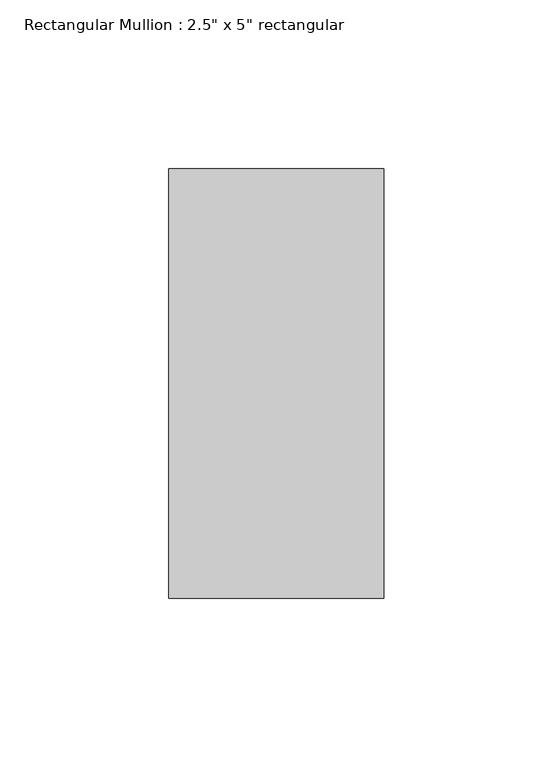
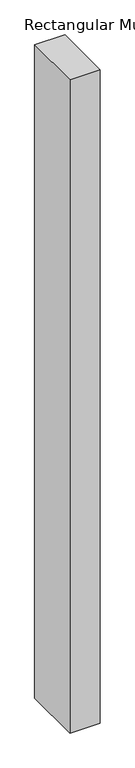
"""IFC4 building model written with IfcOpenShell, lengths in millimetres: member geometry."""

from ifc_helpers import new_model, si_unit, frame, origin, place, context, project, spatial, polyline, outline, extrude, source, transform, mapped, element, save


def member_408948b5(model_context):
    return source(origin(), model_context, "Body", "SweptSolid", [
        extrude(outline(polyline([(0.0, 63.5), (0.0, -63.5), (-63.5, -63.5), (-63.5, 63.5), (0.0, 63.5)])), frame((0.0, 0.0, -1441.7145247), z_axis=(0.0, 0.0, 1.0), x_axis=(1.0, 0.0, 0.0)), (0.0, 0.0, 1.0), 1441.7145247),
    ])


if __name__ == "__main__":
    model = new_model("IFC4")
    model_context = context("Model", 3, world=origin())
    ifc_project = project(units=[si_unit("LENGTHUNIT", "METRE", prefix="MILLI")], contexts=[model_context])
    site = spatial("IfcSite", under=ifc_project)
    building = spatial("IfcBuilding", under=site)
    placement = place(None, origin())
    member_shape = member_408948b5(model_context)
    element("IfcMember", 1, ObjectType="Rectangular Mullion : 2.5\" x 5\" rectangular", at=placement, inside=building, context=model_context, shape_type="MappedRepresentation", body=[
        mapped(member_shape, transform((0.0, 0.0, 0.0), x_axis=(1.0, 0.0, 0.0), y_axis=(0.0, 1.0, 0.0), z_axis=(0.0, 0.0, 1.0))),
    ])
    save(model, "model.ifc")

# Revit data of these elements
# Type "Rectangular Mullion : 2.5\" x 5\" rectangular"
#   built-in parameter 1007304 = 0.416667 (stored number, unit not read)
#   built-in parameter 1007301 = 0.104167 (stored number, unit not read)
#   built-in parameter 1007300 = 0.104167 (stored number, unit not read)
# Element 1 (IfcMember, "Rectangular Mullion : 2.5\" x 5\" rectangular")
#   Materials on its faces: "Aluminum"
# Materials
#   "Aluminum": class "Metal", colour RGB 247 247 247, transparency 0, Description = "Aluminum 6061", Cost = 0
